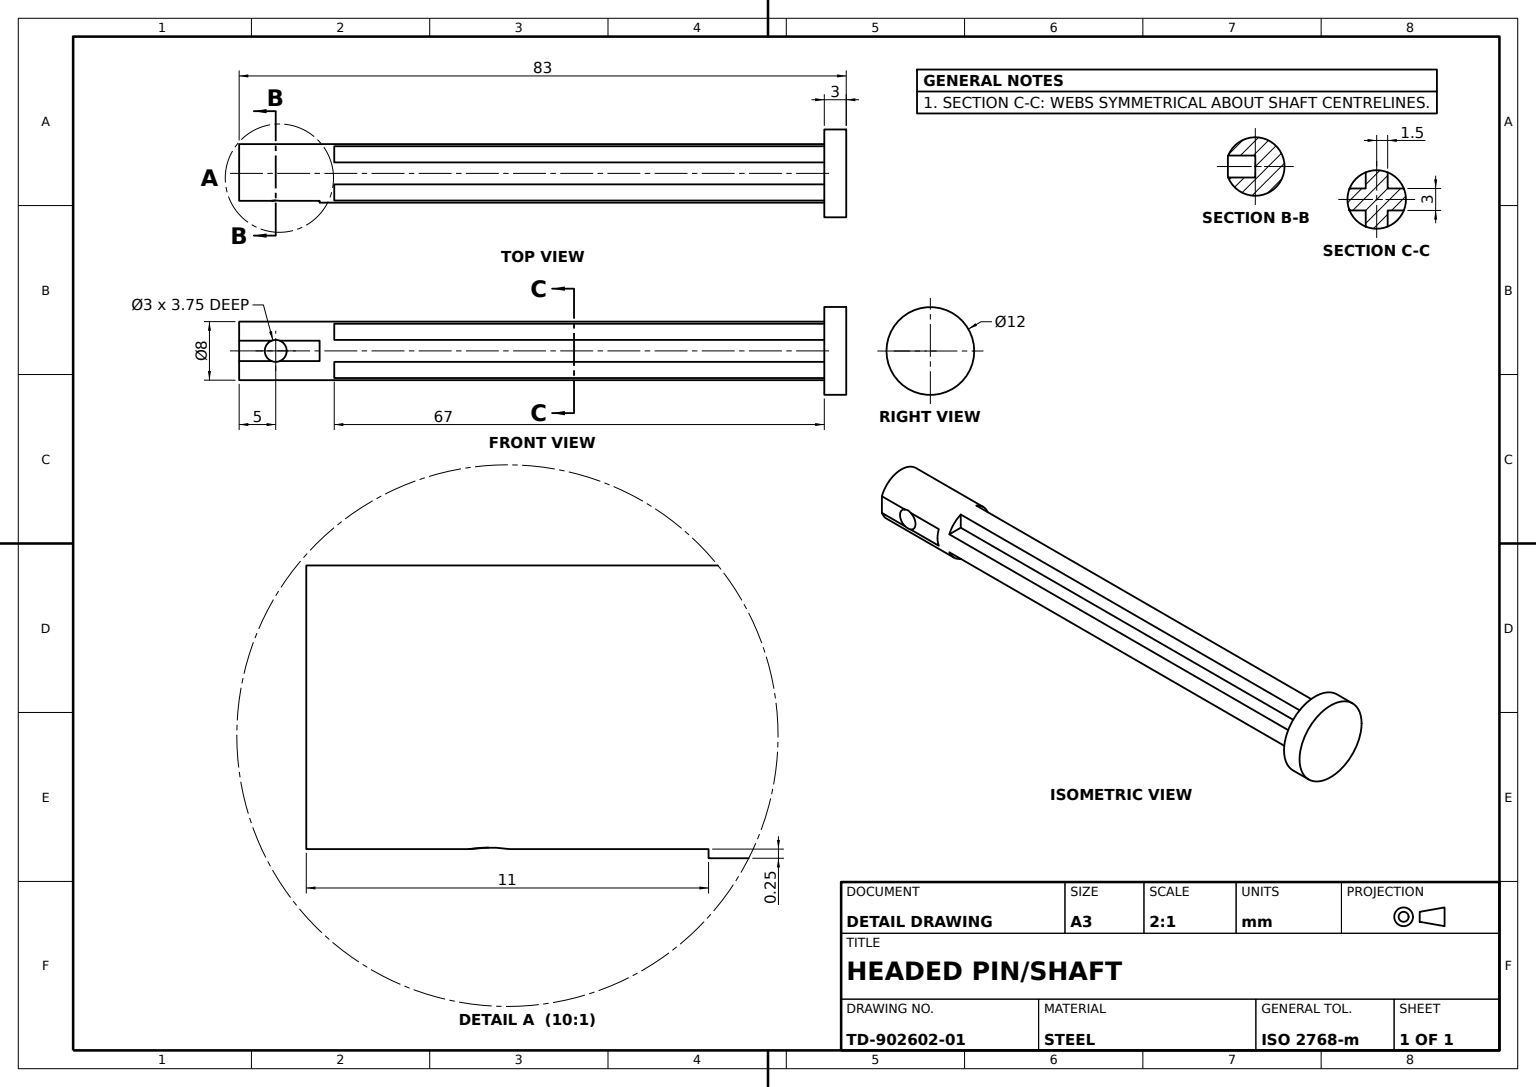
from build123d import *

# Parameters (mm, degrees)
SHANK_PROFILE_8_R           = 4
SHANK_8X80_DEPTH            = 80
SHANK_START                 = -67
SHANK_FLATS_67MM_DEPTH      = 67
HEAD_PROFILE_12_R           = 6
HEAD_12X3_DEPTH             = 3
END_CUT_PROFILE_R           = 1.5
END_POCKET_CUT_4MM_DEPTH    = 4
SKETCH5_4_W                 = 11
SKETCH5_4_H                 = 3
END_RELIEF_CUT_0_25MM_DEPTH = 0.25


with BuildPart() as part:
    # Shank Profile _8 → Shank _8x80 (new body)
    with BuildSketch(Plane(origin=(0, 0, 0), x_dir=(0, 0, -1), z_dir=(1, 0, 0))):
        Circle(SHANK_PROFILE_8_R)
    extrude(amount=SHANK_8X80_DEPTH)

    # Shank Flats Profile → Shank Flats 67mm (cut)
    with BuildSketch(Plane(origin=(80, 0, 0), x_dir=(0, 0, -1), z_dir=(1, 0, 0)).offset(SHANK_START)):
        with BuildLine():
            Line((-1.5, 1.5), (-1.5, 3.708099244))
            ThreePointArc((-1.5, 3.708099244), (-2.828427125, 2.828427125), (-3.708099244, 1.5))
            Line((-3.708099244, 1.5), (-1.5, 1.5))
        make_face()
        with BuildLine():
            Line((1.5, 1.5), (1.5, 3.708099244))
            ThreePointArc((1.5, 3.708099244), (2.828427125, 2.828427125), (3.708099244, 1.5))
            Line((3.708099244, 1.5), (1.5, 1.5))
        make_face()
        with BuildLine():
            Line((1.5, -3.708099244), (1.5, -1.5))
            Line((1.5, -1.5), (3.708099244, -1.5))
            ThreePointArc((3.708099244, -1.5), (2.828427125, -2.828427125), (1.5, -3.708099244))
        make_face()
        with BuildLine():
            Line((-3.708099244, -1.5), (-1.5, -1.5))
            Line((-1.5, -1.5), (-1.5, -3.708099244))
            ThreePointArc((-1.5, -3.708099244), (-2.828427125, -2.828427125), (-3.708099244, -1.5))
        make_face()
    extrude(amount=SHANK_FLATS_67MM_DEPTH, mode=Mode.SUBTRACT)

    # Head Profile _12 → Head _12x3 (add)
    with BuildSketch(Plane(origin=(80, 0, 0), x_dir=(0, 0, -1), z_dir=(1, 0, 0))):
        Circle(HEAD_PROFILE_12_R)
    extrude(amount=HEAD_12X3_DEPTH)

    # End Cut Profile → End Pocket Cut 4mm (cut)
    with BuildSketch(Plane.XY.offset(4)):
        with Locations((5, 0)):
            Circle(END_CUT_PROFILE_R)
    extrude(amount=-END_POCKET_CUT_4MM_DEPTH, mode=Mode.SUBTRACT)

    # Sketch5_4 → End Relief Cut 0.25mm (cut)
    with BuildSketch(Plane.XY.offset(4)):
        with Locations((5.5, 0)):
            Rectangle(SKETCH5_4_W, SKETCH5_4_H)
    extrude(amount=-END_RELIEF_CUT_0_25MM_DEPTH, mode=Mode.SUBTRACT)


solid = part.part
